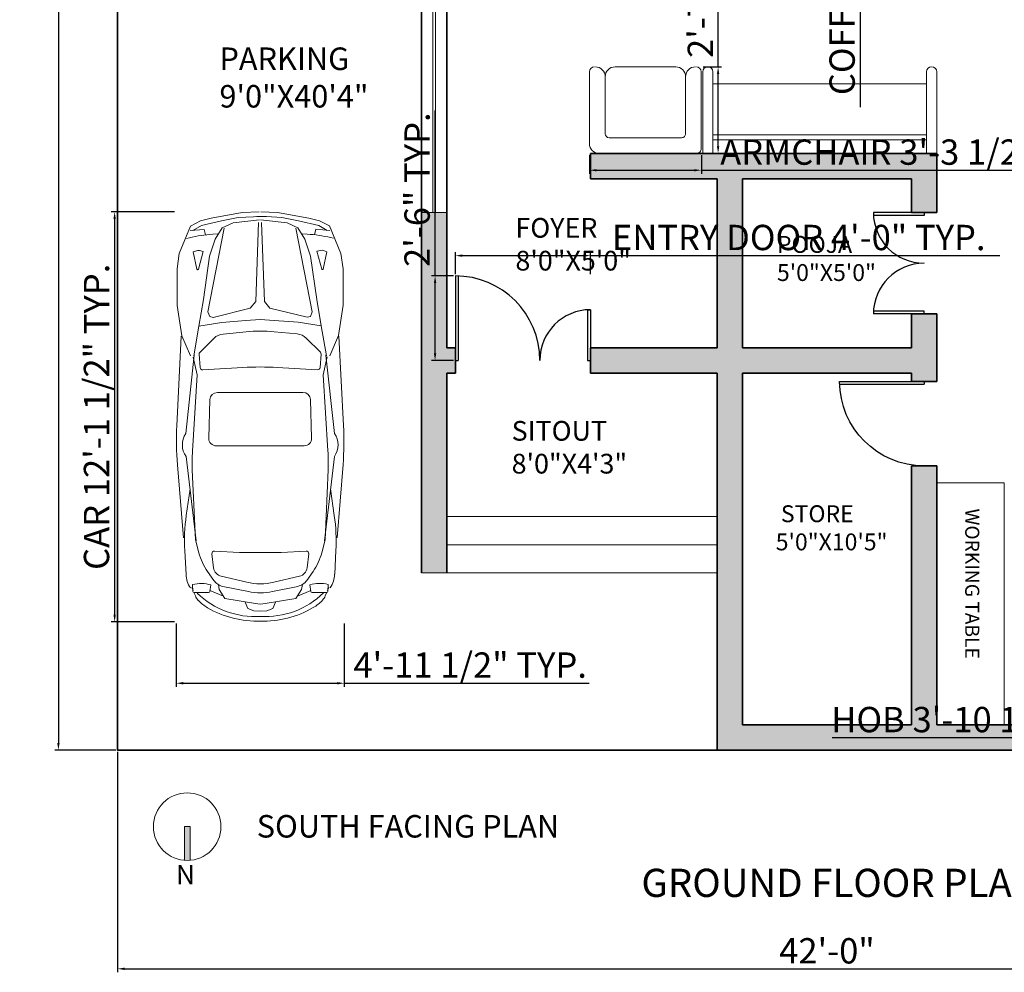
# Model space of a CAD drawing. Units: inches. Extents: x 4606 to 5879, y 1332 to 2209.
# Tile 1 of 7: x 4624 to 4974, y 1332 to 1671. Entities that reach past the tile are written whole.
import ezdxf

# ---------------------------------------------------------------- set-up
doc = ezdxf.new("R2010")
doc.units = ezdxf.units.IN
for name, color, linetype, lineweight in [('A-ANNO-DIMS', 2, 'Continuous', 18), ('A-ANNO-SYMB', 7, 'Continuous', 18), ('A-ANNO-TEXT', 7, 'Continuous', 18), ('A-ANNO-TITL', 7, 'Continuous', 25), ('A-AREA-IDEN', 7, 'Continuous', 18), ('A-DOOR', 4, 'Continuous', 25), ('A-FLOR-CASE', 32, 'Continuous', 18), ('A-FLOR-STRS', 7, 'Continuous', 20), ('A-FURN', 8, 'Continuous', 18), ('A-SITE-PARK', 8, 'Continuous', 13), ('A-WALL', 7, 'Continuous', 35), ('A-WALL-PATT', 252, 'Continuous', 13), ('window', 130, 'Continuous', 18)]:
    doc.layers.add(name, color=color, linetype=linetype, lineweight=lineweight)
doc.styles.get("Standard").update_dxf_attribs({"font": 'arial.ttf'})
doc.dimstyles.new('ISO-25', dxfattribs={"dimtxt": 9, "dimasz": 2.5, "dimexe": 1.25, "dimexo": 0.625, "dimtad": 1, "dimlunit": 3, "dimtxsty": 'Standard', "dimcen": 2.5, "dimadec": 0, "dimazin": 0, "dimtfac": 1, "dimtmove": 0, "dimatfit": 3, "dimfxl": 1, "dimarcsym": 0})

# ---------------------------------------------------------------- blocks, each defined once
blk = doc.blocks.new('D')
for p, q in [((0, 30), (0, 0)), ((1, 29.93), (1, 0)), ((47, 18), (47, 0)), ((47, 18), (48, 18)), ((48, 18), (48, 0)), ((0, 0), (1, 0)), ((47, 0), (48, 0))]:
    blk.add_line(p, q)
for centre, radius, start, end in [((0, 0), 30, 0, 90), ((48, 0), 18, 90, 180)]:
    blk.add_arc(centre, radius, start, end)
blk = doc.blocks.new('D3')
for p, q in [((0, 0), (0, 18)), ((1, 0), (1, 18)), ((35, 0), (35, 18)), ((36, 0), (36, 18)), ((0, 0), (1, 0)), ((36, 0), (35, 0))]:
    blk.add_line(p, q)
for centre, start, end in [((0, 0), 0, 90), ((36, 0), 90, 180)]:
    blk.add_arc(centre, 18, start, end)
blk = doc.blocks.new('sofa-27')
at = {"color": 0, "linetype": 'ByBlock'}
for p, q in [((-0.0591, 0.0591), (-0.0591, 0.4902)), ((0.0945, 0.5198), (0.459, 0.5198)), ((0.6125, 0.0295), (0.6125, 0.4902)), ((0.0354, 0.1181), (0.0354, 0.4607)), ((0.518, 0.1181), (0.518, 0.4607)), ((0.4944, 0.0945), (0.0591, 0.0945)), ((0.583, 0), (0, 0))]:
    blk.add_line(p, q, dxfattribs=at)
for centre, radius, start, end in [((-0.0295, 0.4902), 0.0295, 90, 180), ((-0.0236, 0.4607), 0.0591, 360, 90), ((0.0945, 0.4607), 0.0591, 90, 180), ((0.459, 0.4607), 0.0591, 0, 90), ((0.5771, 0.4607), 0.0591, 90, 180), ((0.583, 0.4902), 0.0295, 0, 90), ((0.0591, 0.1181), 0.0236, 180, 270), ((0.4944, 0.1181), 0.0236, 270, 0), ((0, 0.0591), 0.0591, 180, 270), ((0.583, 0.0295), 0.0295, 270, 0)]:
    blk.add_arc(centre, radius, start, end, dxfattribs=at)
blk = doc.blocks.new('A$C4A3239E3')
for p, q in [((1.2507, 1.6335), (2.1522, 1.6799)), ((1.4425, 1.5023), (2.2313, 1.5881)), ((2.4629, 1.587), (3.3117, 1.4863)), ((2.5445, 1.6742), (3.2816, 1.6148)), ((3.4104, 1.6024), (3.6491, 1.5899)), ((0.1359, 1.4288), (0.1867, 1.515)), ((0.1752, 1.399), (0.1867, 1.5408)), ((0.2661, 1.5794), (0.2592, 1.5495)), ((0.3898, 1.477), (0.4021, 1.5106)), ((0.4021, 1.5106), (0.5754, 1.4741)), ((1.4497, 1.5063), (1.149, 1.4553)), ((1.4612, 1.5146), (1.6407, 1.4739)), ((1.6407, 1.4739), (2.4076, 1.5225)), ((2.597, 1.5244), (3.3012, 1.4943)), ((2.7875, 1.5463), (3.0567, 1.5859)), ((3.3012, 1.4943), (3.4322, 1.4598)), ((3.8218, 1.5205), (3.7519, 1.525)), ((3.7813, 1.5317), (3.8128, 1.5185)), ((3.8334, 1.3629), (3.8334, 1.5081)), ((3.8376, 1.5081), (3.8668, 1.4958)), ((0.0905, 1.2265), (0.1359, 1.4288)), ((0.2308, 1.3867), (0.1752, 1.399)), ((0.3963, 1.4117), (0.388, 1.4492)), ((0.5758, 1.4596), (0.3963, 1.4117)), ((1.2717, 1.3033), (1.4134, 1.4465)), ((1.4329, 1.4538), (1.567, 1.4437)), ((1.59, 1.4175), (1.5668, 1.0125)), ((0.224, 1.314), (0.2207, 1.2655)), ((1.8899, 1.3452), (2.2788, 1.3576)), ((3.4158, 1.3024), (3.4294, 1.0516)), ((3.4434, 1.3284), (3.584, 1.3121)), ((3.6217, 1.372), (3.7108, 1.3099)), ((3.7558, 1.3393), (3.8231, 1.3506)), ((3.8137, 1.3503), (3.8686, 1.2144)), ((0.0565, 1.0588), (0.0905, 1.2265)), ((1.2074, 0.9801), (1.2293, 1.2125)), ((1.8186, 0.4085), (1.8178, 1.2708)), ((2.3557, 1.283), (2.3566, 0.3973)), ((3.6693, 1.236), (3.7299, 0.9762)), ((3.7535, 1.2644), (3.8014, 1.2553)), ((3.7713, 1.2181), (3.8245, 0.9626)), ((3.8014, 1.2553), (3.8941, 1.199)), ((3.8941, 1.199), (3.9452, 0.89)), ((0.0481, 0.9038), (0.0565, 1.0588)), ((3.4294, 1.0516), (3.4292, 0.8428)), ((3.9292, 0.9941), (3.9933, 0.9668)), ((3.9933, 0.9668), (4.0172, 0.906)), ((4.0172, 0.906), (4.0211, 0.842)), ((3.4299, 0.6309), (3.4292, 0.8396)), ((3.8948, 0.4844), (3.9453, 0.7934)), ((4.0174, 0.7775), (4.0211, 0.8416)), ((0.0482, 0.7723), (0.0569, 0.6172)), ((1.2077, 0.6979), (1.23, 0.4656)), ((3.6701, 0.4469), (3.7301, 0.7068)), ((3.772, 0.465), (3.8248, 0.7206)), ((3.9295, 0.6893), (3.9936, 0.7167)), ((3.9936, 0.7167), (4.0174, 0.7775)), ((0.0569, 0.6172), (0.0912, 0.4496)), ((1.5911, 0.2613), (1.5671, 0.6662)), ((3.4167, 0.38), (3.4299, 0.6309)), ((0.0912, 0.4496), (0.1371, 0.2474)), ((0.2249, 0.3624), (0.2215, 0.4109)), ((3.7543, 0.4187), (3.8022, 0.4279)), ((3.8022, 0.4279), (3.8948, 0.4844)), ((3.8147, 0.3328), (3.8693, 0.4688)), ((1.2726, 0.3749), (1.4146, 0.232)), ((1.8909, 0.3342), (2.2798, 0.3226)), ((3.4444, 0.354), (3.585, 0.3707)), ((3.6228, 0.3107), (3.7117, 0.3731)), ((3.7568, 0.3438), (3.8241, 0.3326)), ((3.8345, 0.3203), (3.8347, 0.1751)), ((0.1371, 0.2474), (0.188, 0.1613)), ((0.2318, 0.2897), (0.1763, 0.2773)), ((0.1763, 0.2773), (0.1881, 0.1355)), ((0.3975, 0.2651), (0.3892, 0.2275)), ((0.3911, 0.1998), (0.4034, 0.1661)), ((0.5771, 0.2174), (0.3975, 0.2651)), ((0.4034, 0.1661), (0.5767, 0.203)), ((1.451, 0.1722), (1.1502, 0.2226)), ((1.4341, 0.2247), (1.5682, 0.235)), ((1.4625, 0.1639), (1.6419, 0.205)), ((1.6419, 0.205), (2.4089, 0.1579)), ((3.3024, 0.1879), (3.4334, 0.2226)), ((0.2676, 0.0971), (0.2606, 0.127)), ((1.4438, 0.1762), (2.2328, 0.0919)), ((2.4644, 0.0936), (3.313, 0.1959)), ((2.5984, 0.1564), (3.3024, 0.1879)), ((2.7889, 0.1349), (3.0581, 0.0958)), ((3.8231, 0.1627), (3.7532, 0.1581)), ((3.7826, 0.1514), (3.8141, 0.1647)), ((3.8389, 0.1752), (3.8681, 0.1875)), ((1.2522, 0.0446), (2.1538, 0)), ((2.5461, 0.0065), (3.2831, 0.0673)), ((3.4119, 0.0799), (3.6506, 0.0929))]:
    blk.add_line(p, q)
for points in [[(0, 0.8478), (0.0053, 1.0159), (0.0622, 1.3298), (0.0905, 1.4375), (0.1412, 1.5365), (0.4188, 1.6529), (0.572, 1.6743), (0.9399, 1.6743), (1.2458, 1.627), (1.4497, 1.5408)], [(0.0815, 0.8439), (0.1088, 1.11), (0.1609, 1.2182), (0.2737, 1.2906), (0.4463, 1.3472), (0.8811, 1.4091), (1.149, 1.4553), (1.1121, 1.224), (1.0933, 0.9813), (1.085, 0.8389)], [(0.1644, 1.198), (1.0072, 1.3636), (1.0537, 1.3462), (1.0619, 1.3117), (0.9706, 0.937), (0.9035, 0.8818), (0.106, 0.853)], [(0, 0.8281), (0.0056, 0.6601), (0.0632, 0.3462), (0.0916, 0.2386), (0.1426, 0.1398), (0.4204, 0.0239), (0.5737, 0.0028), (0.9415, 0.0032), (1.2473, 0.0511), (1.4511, 0.1377)], [(0.0815, 0.8322), (0.1094, 0.5662), (0.1616, 0.4581), (0.2746, 0.3859), (0.4473, 0.3296), (0.8822, 0.2683), (1.1502, 0.2226), (1.1128, 0.4539), (1.0936, 0.6965), (1.085, 0.8389)], [(0.1651, 0.4782), (1.0082, 0.314), (1.0547, 0.3316), (1.0628, 0.366), (0.9708, 0.7406), (0.9036, 0.7957), (0.1061, 0.8232)]]:
    blk.add_lwpolyline(points)
for centre, radius, start, end in [((2.3053, -1.296), 2.9798, 85.39524, 92.94517), ((2.3463, 1.4226), 0.2016, 54.64918, 124.77695), ((3.3168, -0.183), 1.7879, 86.99981, 98.3676), ((3.6355, 1.3122), 0.278, 57.32995, 87.18237), ((1.7104, 1.2122), 1.4899, 166.91658, 176.08111), ((2.5206, -0.2618), 1.7879, 87.54913, 93.62371), ((4.0973, 1.4394), 0.3558, 166.09608, 196.35351), ((3.821, 1.5081), 0.0124, 0, 86.33043), ((3.8091, 1.3584), 0.149, 46.38363, 67.20138), ((0.4365, 1.46), 0.0497, 159.97873, 192.53841), ((0.5739, 1.4668), 0.00745, 284.96001, 78.11246), ((1.431, 1.429), 0.0248, 85.71507, 135.30465), ((1.5652, 1.4189), 0.0248, 356.72561, 85.71507), ((3.2805, 0.8834), 0.596, 55.07004, 75.25506), ((3.2466, 0.8963), 0.8285, 356.24509, 44.51945), ((3.6181, 1.158), 0.4258, 30.45768, 46.38363), ((1.3776, 1.1985), 0.149, 135.30465, 174.62136), ((1.8923, 1.2708), 0.0745, 91.82012, 179.9989), ((2.2812, 1.2831), 0.0745, 359.92446, 91.82012), ((3.4406, 1.3037), 0.0248, 83.37601, 183.11504), ((3.5726, 1.2134), 0.0993, 13.12265, 83.37601), ((3.6254, 1.1877), 0.149, 11.76937, 55.07004), ((3.821, 1.3629), 0.0124, 279.60772, 0), ((3.1325, 0.8724), 0.9892, 358.06945, 30.45768), ((4.5417, 0.8423), 2.9798, 176.72561, 183.38736), ((1.2382, 0.8392), 1.1919, 176.89416, 183.21881), ((2.6908, 0.8405), 1.4899, 174.62136, 185.49162), ((3.1495, 0.8409), 0.596, 346.99033, 13.12265), ((3.2411, 0.841), 0.596, 348.3436, 11.76937), ((3.2467, 0.7858), 0.8285, 315.59352, 3.86789), ((3.6512, 0.8414), 0.298, 350.72464, 9.38834), ((3.1326, 0.8094), 0.9892, 329.65529, 2.04353), ((1.3783, 0.4799), 0.149, 185.49162, 224.80833), ((1.8931, 0.4086), 0.0745, 180.11408, 268.29286), ((2.2821, 0.397), 0.0745, 268.29286, 0.18852), ((3.5733, 0.4693), 0.0993, 276.73697, 346.99033), ((3.6261, 0.4951), 0.149, 305.04293, 348.3436), ((1.7111, 0.4671), 1.4899, 184.03187, 193.1964), ((3.4415, 0.3787), 0.0248, 176.99794, 276.73697), ((3.2806, 0.7987), 0.596, 284.85791, 305.04293), ((4.0985, 0.2443), 0.3558, 163.75946, 194.01689), ((3.822, 0.3203), 0.0124, 0.11298, 80.50526), ((3.6188, 0.5248), 0.4258, 313.72935, 329.65529), ((0.4377, 0.2169), 0.0497, 167.57457, 200.13424), ((0.5752, 0.2102), 0.00745, 282.00051, 75.15297), ((1.4322, 0.2495), 0.0248, 224.80833, 274.3979), ((1.5663, 0.2598), 0.0248, 274.3979, 3.38736), ((3.8101, 0.3247), 0.149, 292.9116, 313.72935), ((2.5184, 1.9425), 1.7879, 266.48926, 272.56385), ((3.6364, 0.3706), 0.278, 272.9306, 302.78303), ((3.8223, 0.1751), 0.0124, 273.78255, 0.11298), ((2.3011, 2.9762), 2.9798, 267.1678, 274.71773), ((2.3474, 0.2577), 0.2016, 235.33603, 305.46379), ((3.3148, 1.8652), 1.7879, 261.74537, 273.11317)]:
    blk.add_arc(centre, radius, start, end)
blk = doc.blocks.new('D2')
for p, q in [((0, 30), (0, 0)), ((1, 30), (1, 0)), ((0, 0), (1, 0))]:
    blk.add_line(p, q)
blk.add_arc((0, 0), 30, 0, 90)
blk = doc.blocks.new('*D24')
at = {"layer": 'A-ANNO-DIMS', "color": 0, "lineweight": -2, "transparency": 16777216}
for p, q in [((4658.23, 2081.24), (4636.6, 2081.24)), ((4637.85, 2078.74), (4637.85, 1413.74)), ((4658.23, 1411.24), (4636.6, 1411.24))]:
    blk.add_line(p, q, dxfattribs=at)
at = {"layer": 'A-ANNO-DIMS', "color": 0, "transparency": 16777216}
for points in [[(4637.43, 2078.74), (4638.26, 2078.74), (4637.85, 2081.24)], [(4637.43, 1413.74), (4638.26, 1413.74), (4637.85, 1411.24)]]:
    blk.add_solid(points, dxfattribs=at)
at = {"layer": 'Defpoints', "color": 0, "transparency": 16777216}
for p in [(4658.85, 2081.24), (4637.85, 1411.24), (4658.85, 1411.24)]:
    blk.add_point(p, dxfattribs=at)
at = {"layer": 'A-ANNO-DIMS', "color": 0, "transparency": 16777216, "insert": (4632.62, 1746.24), "char_height": 9, "attachment_point": 5, "rotation": 90}
blk.add_mtext('55\'-10"', dxfattribs=at)
blk = doc.blocks.new('GLAZING-72IN')
for p, q in [((0, 0), (0, 72)), ((1, 0), (1, 72))]:
    blk.add_line(p, q)
blk = doc.blocks.new('NORTH-ARROW')
at = {"transparency": 33554687}
h = blk.add_hatch(color=256, dxfattribs=at)
h.dxf.hatch_style = 1
h.paths.add_polyline_path([(13, 20.5), (11, 20.5), (11, 8.55, 0.020861), (12, 8.5, 0.020861), (13, 8.55)])
for p, q in [((11, 8.5), (11, 20.5)), ((11, 20.5), (13, 20.5)), ((13, 20.5), (13, 8.55))]:
    blk.add_line(p, q)
blk.add_circle((12, 20.5), 12)
blk.add_text('N', height=6.9).set_placement((7.98, 0))
blk = doc.blocks.new('*D77')
at = {"layer": 'A-ANNO-DIMS', "color": 0, "lineweight": -2, "transparency": 16777216}
for p, q in [((4778.85, 1580.36), (4778.85, 1588.19)), ((4826.85, 1580.36), (4826.85, 1588.19)), ((4781.35, 1586.94), (4824.35, 1586.94)), ((4826.85, 1586.94), (4972.3, 1586.94))]:
    blk.add_line(p, q, dxfattribs=at)
at = {"layer": 'A-ANNO-DIMS', "color": 0, "transparency": 16777216}
for points in [[(4781.35, 1587.36), (4781.35, 1586.52), (4778.85, 1586.94)], [(4824.35, 1587.36), (4824.35, 1586.52), (4826.85, 1586.94)]]:
    blk.add_solid(points, dxfattribs=at)
at = {"layer": 'Defpoints', "color": 0, "transparency": 16777216}
for p in [(4826.85, 1586.94), (4778.85, 1579.74), (4826.85, 1579.74)]:
    blk.add_point(p, dxfattribs=at)
at = {"layer": 'A-ANNO-DIMS', "color": 0, "transparency": 16777216, "insert": (4900.83, 1592.22), "char_height": 9, "attachment_point": 5}
blk.add_mtext('ENTRY DOOR 4\'-0" TYP.', dxfattribs=at)
blk = doc.blocks.new('*D78')
at = {"layer": 'A-ANNO-DIMS', "color": 0, "lineweight": -2, "transparency": 16777216}
for p, q in [((4771.65, 1579.74), (4771.65, 1638.5)), ((4778.23, 1579.74), (4770.4, 1579.74)), ((4771.65, 1552.24), (4771.65, 1577.24)), ((4778.23, 1549.74), (4770.4, 1549.74))]:
    blk.add_line(p, q, dxfattribs=at)
at = {"layer": 'A-ANNO-DIMS', "color": 0, "transparency": 16777216}
for points in [[(4771.23, 1577.24), (4772.07, 1577.24), (4771.65, 1579.74)], [(4771.23, 1552.24), (4772.07, 1552.24), (4771.65, 1549.74)]]:
    blk.add_solid(points, dxfattribs=at)
at = {"layer": 'Defpoints', "color": 0, "transparency": 16777216}
for p in [(4771.65, 1579.74), (4778.85, 1579.74), (4778.85, 1549.74)]:
    blk.add_point(p, dxfattribs=at)
at = {"layer": 'A-ANNO-DIMS', "color": 0, "transparency": 16777216, "insert": (4766.43, 1610.37), "char_height": 9, "attachment_point": 5, "rotation": 90}
blk.add_mtext('2\'-6" TYP.', dxfattribs=at)
blk = doc.blocks.new('*D87')
at = {"layer": 'A-ANNO-DIMS', "color": 0, "lineweight": -2, "transparency": 16777216}
for p, q in [((4826.48, 1622.61), (4826.48, 1616.03)), ((4866.23, 1622.61), (4866.23, 1616.03)), ((4828.98, 1617.28), (4863.73, 1617.28)), ((4866.23, 1617.28), (5016.88, 1617.28))]:
    blk.add_line(p, q, dxfattribs=at)
at = {"layer": 'A-ANNO-DIMS', "color": 0, "transparency": 16777216}
for points in [[(4828.98, 1617.69), (4828.98, 1616.86), (4826.48, 1617.28)], [(4863.73, 1617.69), (4863.73, 1616.86), (4866.23, 1617.28)]]:
    blk.add_solid(points, dxfattribs=at)
at = {"layer": 'Defpoints', "color": 0, "transparency": 16777216}
for p in [(4826.48, 1623.24), (4866.23, 1623.24), (4866.23, 1617.28)]:
    blk.add_point(p, dxfattribs=at)
at = {"layer": 'A-ANNO-DIMS', "color": 0, "transparency": 16777216, "insert": (4942.8, 1622.56), "char_height": 9, "attachment_point": 5}
blk.add_mtext('ARMCHAIR 3\'-3 1/2" TYP.', dxfattribs=at)
blk = doc.blocks.new('*D88')
at = {"layer": 'A-ANNO-DIMS', "color": 0, "lineweight": -2, "transparency": 16777216}
for p, q in [((4872.19, 1654), (4872.19, 1712.76)), ((4866.85, 1654), (4873.44, 1654)), ((4872.19, 1625.74), (4872.19, 1651.5)), ((4866.85, 1623.24), (4873.44, 1623.24))]:
    blk.add_line(p, q, dxfattribs=at)
at = {"layer": 'A-ANNO-DIMS', "color": 0, "transparency": 16777216}
for points in [[(4871.77, 1651.5), (4872.6, 1651.5), (4872.19, 1654)], [(4871.77, 1625.74), (4872.6, 1625.74), (4872.19, 1623.24)]]:
    blk.add_solid(points, dxfattribs=at)
at = {"layer": 'Defpoints', "color": 0, "transparency": 16777216}
for p in [(4866.23, 1654), (4872.19, 1654), (4866.23, 1623.24)]:
    blk.add_point(p, dxfattribs=at)
at = {"layer": 'A-ANNO-DIMS', "color": 0, "transparency": 16777216, "insert": (4867.04, 1684.63), "char_height": 9, "attachment_point": 5, "rotation": 90}
blk.add_mtext('2\'-7" TYP.', dxfattribs=at)
blk = doc.blocks.new('*D103')
at = {"layer": 'A-ANNO-DIMS', "color": 0, "lineweight": -2, "transparency": 16777216}
for p, q in [((4679.05, 1602.48), (4656.58, 1602.48)), ((4657.83, 1599.98), (4657.83, 1459.37)), ((4679.05, 1456.87), (4656.58, 1456.87))]:
    blk.add_line(p, q, dxfattribs=at)
at = {"layer": 'A-ANNO-DIMS', "color": 0, "transparency": 16777216}
for points in [[(4657.41, 1599.98), (4658.25, 1599.98), (4657.83, 1602.48)], [(4657.41, 1459.37), (4658.25, 1459.37), (4657.83, 1456.87)]]:
    blk.add_solid(points, dxfattribs=at)
at = {"layer": 'Defpoints', "color": 0, "transparency": 16777216}
for p in [(4679.67, 1602.48), (4657.83, 1456.87), (4679.67, 1456.87)]:
    blk.add_point(p, dxfattribs=at)
at = {"layer": 'A-ANNO-DIMS', "color": 0, "transparency": 16777216, "insert": (4652.55, 1529.68), "char_height": 9, "attachment_point": 5, "rotation": 90}
blk.add_mtext('CAR 12\'-1 1/2" TYP.', dxfattribs=at)
blk = doc.blocks.new('*D104')
at = {"layer": 'A-ANNO-DIMS', "color": 0, "lineweight": -2, "transparency": 16777216}
for p, q in [((4679.67, 1456.25), (4679.67, 1433.78)), ((4739.4, 1456.25), (4739.4, 1433.78)), ((4682.17, 1435.03), (4736.9, 1435.03)), ((4739.4, 1435.03), (4826.33, 1435.03))]:
    blk.add_line(p, q, dxfattribs=at)
at = {"layer": 'A-ANNO-DIMS', "color": 0, "transparency": 16777216}
for points in [[(4682.17, 1435.45), (4682.17, 1434.61), (4679.67, 1435.03)], [(4736.9, 1435.45), (4736.9, 1434.61), (4739.4, 1435.03)]]:
    blk.add_solid(points, dxfattribs=at)
at = {"layer": 'Defpoints', "color": 0, "transparency": 16777216}
for p in [(4679.67, 1456.87), (4739.4, 1456.87), (4739.4, 1435.03)]:
    blk.add_point(p, dxfattribs=at)
at = {"layer": 'A-ANNO-DIMS', "color": 0, "transparency": 16777216, "insert": (4784.11, 1440.31), "char_height": 9, "attachment_point": 5}
blk.add_mtext('4\'-11 1/2" TYP.', dxfattribs=at)
blk = doc.blocks.new('*D105')
at = {"layer": 'A-ANNO-DIMS', "color": 0, "lineweight": -2, "transparency": 16777216}
for p, q in [((4927.48, 1801.23), (4921.43, 1801.23)), ((4922.68, 1798.73), (4922.68, 1767.59)), ((4927.48, 1765.09), (4921.43, 1765.09)), ((4922.68, 1765.09), (4922.68, 1639.71))]:
    blk.add_line(p, q, dxfattribs=at)
at = {"layer": 'A-ANNO-DIMS', "color": 0, "transparency": 16777216}
for points in [[(4922.27, 1798.73), (4923.1, 1798.73), (4922.68, 1801.23)], [(4922.27, 1767.59), (4923.1, 1767.59), (4922.68, 1765.09)]]:
    blk.add_solid(points, dxfattribs=at)
at = {"layer": 'Defpoints', "color": 0, "transparency": 16777216}
for p in [(4928.1, 1801.23), (4922.68, 1765.09), (4928.1, 1765.09)]:
    blk.add_point(p, dxfattribs=at)
at = {"layer": 'A-ANNO-DIMS', "color": 0, "transparency": 16777216, "insert": (4917.4, 1701.15), "char_height": 9, "attachment_point": 5, "rotation": 90}
blk.add_mtext('COFFEE TABLE 3\'-0"', dxfattribs=at)
blk = doc.blocks.new('*D109')
at = {"layer": 'A-ANNO-DIMS', "color": 0, "lineweight": -2, "transparency": 16777216}
for p, q in [((4998.57, 1422), (4998.57, 1414.41)), ((5045.02, 1422), (5045.02, 1414.41)), ((4998.57, 1415.66), (4912.68, 1415.66)), ((5042.52, 1415.66), (5001.07, 1415.66))]:
    blk.add_line(p, q, dxfattribs=at)
at = {"layer": 'A-ANNO-DIMS', "color": 0, "transparency": 16777216}
for points in [[(5001.07, 1416.08), (5001.07, 1415.25), (4998.57, 1415.66)], [(5042.52, 1416.08), (5042.52, 1415.25), (5045.02, 1415.66)]]:
    blk.add_solid(points, dxfattribs=at)
at = {"layer": 'Defpoints', "color": 0, "transparency": 16777216}
for p in [(4998.57, 1422.63), (5045.02, 1422.63), (4998.57, 1415.66)]:
    blk.add_point(p, dxfattribs=at)
at = {"layer": 'A-ANNO-DIMS', "color": 0, "transparency": 16777216, "insert": (4954.38, 1420.95), "char_height": 9, "attachment_point": 5}
blk.add_mtext('HOB 3\'-10 1/2"', dxfattribs=at)
blk = doc.blocks.new('*D113')
at = {"layer": 'A-ANNO-DIMS', "color": 0, "lineweight": -2, "transparency": 16777216}
for p, q in [((4658.85, 1410.61), (4658.85, 1332.33)), ((5162.85, 1410.61), (5162.85, 1332.33)), ((4661.35, 1333.58), (5160.35, 1333.58))]:
    blk.add_line(p, q, dxfattribs=at)
at = {"layer": 'A-ANNO-DIMS', "color": 0, "transparency": 16777216}
for points in [[(4661.35, 1334), (4661.35, 1333.16), (4658.85, 1333.58)], [(5160.35, 1334), (5160.35, 1333.16), (5162.85, 1333.58)]]:
    blk.add_solid(points, dxfattribs=at)
at = {"layer": 'Defpoints', "color": 0, "transparency": 16777216}
for p in [(4658.85, 1411.24), (5162.85, 1411.24), (5162.85, 1333.58)]:
    blk.add_point(p, dxfattribs=at)
at = {"layer": 'A-ANNO-DIMS', "color": 0, "transparency": 16777216, "insert": (4910.85, 1338.8), "char_height": 9, "attachment_point": 5}
blk.add_mtext('42\'-0"', dxfattribs=at)

msp = doc.modelspace()

# ---------------------------------------------------------------- hatches: boundary and pattern name
at = {"layer": 'A-WALL-PATT', "transparency": 33554687}
h = msp.add_hatch(color=256, dxfattribs=at)
h.dxf.hatch_style = 1
h.paths.add_polyline_path([(4715.85, 2081.239), (4658.85, 2081.239), (4658.85, 2054.239), (4667.85, 2054.239), (4667.85, 2072.239), (4715.85, 2072.239)])
h.paths.add_polyline_path([(4868.85, 2081.239), (4787.85, 2081.239), (4787.85, 2072.239), (4835.85, 2072.239), (4835.85, 1955.239), (4844.85, 1955.239), (4844.85, 1970.239), (4850.85, 1970.239), (4850.85, 1976.239), (4844.85, 1976.239), (4844.85, 2072.239), (4868.85, 2072.239)])
h.paths.add_polyline_path([(4940.85, 2081.239), (4892.85, 2081.239), (4892.85, 2072.239), (4916.85, 2072.239), (4916.85, 1976.239), (4880.85, 1976.239), (4880.85, 1970.239), (4916.85, 1970.239), (4916.85, 1904.239), (4844.85, 1904.239), (4844.85, 1925.239), (4835.85, 1925.239), (4835.85, 1904.239), (4832.85, 1904.239), (4832.85, 1895.239), (4919.85, 1895.239), (4991.85, 1895.239), (4991.85, 1904.239), (4988.85, 1904.239), (4988.85, 1925.239), (4982.85, 1925.239), (4982.85, 1904.239), (4922.85, 1904.239), (4922.85, 1970.239), (4946.85, 1970.239), (4946.85, 1976.239), (4922.85, 1976.239), (4922.85, 2072.239), (4940.85, 2072.239)])
h.paths.add_polyline_path([(5021.85, 2081.239), (4964.85, 2081.239), (4964.85, 2072.239), (4982.85, 2072.239), (4982.85, 1976.239), (4976.85, 1976.239), (4976.85, 1970.239), (4982.85, 1970.239), (4982.85, 1955.239), (4988.85, 1955.239), (4988.85, 2072.239), (5021.85, 2072.239)])
h.paths.add_polyline_path([(5135.85, 2081.239), (5093.85, 2081.239), (5093.85, 2072.239), (5126.85, 2072.239), (5126.85, 2054.239), (5135.85, 2054.239)])
h.paths.add_polyline_path([(5135.85, 2006.239), (5126.85, 2006.239), (5126.85, 1976.239), (5135.85, 1976.239)])
h.paths.add_polyline_path([(5135.85, 1928.239), (5126.85, 1928.239), (5126.85, 1904.239), (5027.85, 1904.239), (5027.85, 1895.239), (5126.85, 1895.239), (5126.85, 1871.239), (5135.85, 1871.239)])
h.paths.add_polyline_path([(4796.85, 1904.239), (4667.85, 1904.239), (4667.85, 1922.239), (4658.85, 1922.239), (4658.85, 1895.239), (4766.85, 1895.239), (4766.85, 1674.239), (4775.85, 1674.239), (4775.85, 1895.239), (4796.85, 1895.239)])
h.paths.add_polyline_path([(4667.85, 2006.239), (4658.85, 2006.239), (4658.85, 1970.239), (4667.85, 1970.239)])
h.paths.add_polyline_path([(4880.85, 1545.239), (4940.85, 1545.239), (4940.85, 1542.239), (4949.85, 1542.239), (4949.85, 1566.239), (4940.85, 1566.239), (4940.85, 1554.239), (4880.85, 1554.239), (4880.85, 1614.239), (4940.85, 1614.239), (4940.85, 1602.239), (4949.85, 1602.239), (4949.85, 1623.239), (4866.739, 1623.239), (4826.85, 1623.239), (4826.85, 1614.239), (4871.85, 1614.239), (4871.85, 1554.239), (4826.85, 1554.239), (4826.85, 1545.239), (4871.85, 1545.239), (4871.85, 1411.239), (4997.85, 1411.239), (4997.85, 1420.239), (4949.85, 1420.239), (4949.85, 1512.239), (4940.85, 1512.239), (4940.85, 1420.239), (4880.85, 1420.239)])
h.paths.add_polyline_path([(5102.85, 1446.239), (5093.85, 1446.239), (5093.85, 1420.239), (5045.85, 1420.239), (5045.85, 1411.239), (5102.85, 1411.239)])
h.paths.add_polyline_path([(5102.85, 1591.739), (5093.85, 1591.739), (5093.85, 1542.239), (5102.85, 1542.239)])
h.paths.add_polyline_path([(5135.85, 1691.239), (5126.85, 1691.239), (5126.85, 1673.239), (5030.85, 1673.239), (5030.85, 1676.239), (5021.85, 1676.239), (5021.85, 1673.239), (5003.85, 1673.239), (5003.85, 1664.239), (5093.85, 1664.239), (5093.85, 1639.739), (5102.85, 1639.739), (5102.85, 1664.239), (5135.85, 1664.239)])
h.paths.add_polyline_path([(5135.85, 1823.239), (5126.85, 1823.239), (5126.85, 1799.239), (5028.85, 1799.239), (5028.85, 1790.239), (5057.85, 1790.239), (5057.85, 1784.239), (5066.85, 1784.239), (5066.85, 1790.239), (5126.85, 1790.239), (5126.85, 1742.239), (5066.85, 1742.239), (5066.85, 1748.239), (5057.85, 1748.239), (5057.85, 1742.239), (5021.85, 1742.239), (5021.85, 1706.239), (5030.85, 1706.239), (5030.85, 1733.239), (5126.85, 1733.239), (5126.85, 1715.239), (5135.85, 1715.239)])
h.paths.add_polyline_path([(4775.85, 1602.239), (4766.85, 1602.239), (4766.85, 1474.239), (4775.85, 1474.239), (4775.85, 1545.239), (4778.85, 1545.239), (4778.85, 1554.239), (4775.85, 1554.239)])
h.paths.add_polyline_path([(4692.58, 1635.003), (4749.356, 1635.003), (4749.356, 1665.418), (4692.58, 1665.418)], flags=9)

# ---------------------------------------------------------------- linework, layer by layer
at = {"layer": 'A-FLOR-CASE'}
for q in [(4949.85, 1506.239), (4973.85, 1420.239)]:
    msp.add_line((4973.85, 1506.239), q, dxfattribs=at)
at = {"layer": 'A-FLOR-STRS'}
for p, q in [((4775.85, 1494.239), (4871.85, 1494.239)), ((4775.85, 1484.239), (4871.85, 1484.239)), ((4766.85, 1474.239), (4871.85, 1474.239))]:
    msp.add_line(p, q, dxfattribs=at)
at = {"layer": 'A-FURN'}
for p, q in [((4866.739, 1652.26), (4866.739, 1623.239)), ((4870.367, 1623.239), (4870.367, 1652.26)), ((4946.222, 1652.26), (4946.222, 1623.239)), ((4949.85, 1652.26), (4949.85, 1623.239)), ((4946.222, 1648.026), (4870.367, 1648.026)), ((4870.367, 1629.888), (4946.222, 1629.888)), ((4870.367, 1628.074), (4946.222, 1628.074)), ((4949.85, 1623.239), (4866.739, 1623.239))]:
    msp.add_line(p, q, dxfattribs=at)
for centre in [(4868.553, 1652.26), (4948.036, 1652.26)]:
    msp.add_arc(centre, 1.814, 0, 180, dxfattribs=at)
at = {"layer": 'A-WALL'}
for p, q in [((4766.85, 1895.239), (4766.85, 1474.239)), ((4775.85, 1895.239), (4775.85, 1554.239)), ((4826.85, 1623.239), (4949.85, 1623.239)), ((4826.85, 1623.239), (4826.85, 1614.239)), ((4949.85, 1623.239), (4949.85, 1602.239)), ((4826.85, 1614.239), (4871.85, 1614.239)), ((4871.85, 1614.239), (4871.85, 1554.239)), ((4880.85, 1614.239), (4880.85, 1554.239)), ((4880.85, 1614.239), (4940.85, 1614.239)), ((4940.85, 1614.239), (4940.85, 1602.239)), ((4940.85, 1602.239), (4949.85, 1602.239)), ((4940.85, 1566.239), (4949.85, 1566.239)), ((4940.85, 1566.239), (4940.85, 1554.239)), ((4949.85, 1566.239), (4949.85, 1542.239)), ((4775.85, 1554.239), (4778.85, 1554.239)), ((4778.85, 1554.239), (4778.85, 1545.239)), ((4826.85, 1554.239), (4871.85, 1554.239)), ((4826.85, 1554.239), (4826.85, 1545.239)), ((4880.85, 1554.239), (4940.85, 1554.239)), ((4775.85, 1545.239), (4778.85, 1545.239)), ((4775.85, 1545.239), (4775.85, 1474.239)), ((4826.85, 1545.239), (4871.85, 1545.239)), ((4871.85, 1545.239), (4871.85, 1411.239)), ((4880.85, 1545.239), (4940.85, 1545.239)), ((4880.85, 1545.239), (4880.85, 1420.239)), ((4940.85, 1545.239), (4940.85, 1542.239)), ((4940.85, 1542.239), (4949.85, 1542.239)), ((4940.85, 1512.239), (4949.85, 1512.239)), ((4940.85, 1512.239), (4940.85, 1420.239)), ((4949.85, 1512.239), (4949.85, 1420.239)), ((4880.85, 1420.239), (4940.85, 1420.239)), ((4949.85, 1420.239), (5093.85, 1420.239))]:
    msp.add_line(p, q, dxfattribs=at)
msp.add_lwpolyline([(5135.85, 1664.239), (5135.85, 2081.239), (4658.85, 2081.239), (4658.85, 1411.239), (5102.85, 1411.239)], dxfattribs=at)
at = {"layer": 'window'}
msp.add_line((4766.85, 1602.239), (4775.85, 1602.239), dxfattribs=at)

# ---------------------------------------------------------------- block references
at = {"layer": 'A-ANNO-SYMB'}
msp.add_blockref('NORTH-ARROW', (4671.599, 1363.576), dxfattribs=at)
at = {"layer": 'A-DOOR', "rotation": 90}
msp.add_blockref('D3', (4945.35, 1566.239), dxfattribs=at)
at = {"layer": 'A-DOOR'}
msp.add_blockref('D', (4778.85, 1549.739), dxfattribs=at)
at = {"layer": 'A-DOOR', "xscale": -1, "rotation": 90}
msp.add_blockref('D2', (4945.35, 1542.239), dxfattribs=at)
at = {"layer": 'A-FURN', "xscale": 59.17827105340016, "yscale": 59.17827105340016, "zscale": 59.17827105340016, "rotation": 359.9999999999668}
msp.add_blockref('sofa-27', (4829.977, 1623.239), dxfattribs=at)
at = {"layer": 'A-SITE-PARK', "xscale": 35.27598425228, "yscale": 35.27598425228, "zscale": 35.27598425228, "rotation": 270}
msp.add_blockref('A$C4A3239E3', (4679.899, 1602.485), dxfattribs=at)
at = {"layer": 'window'}
msp.add_blockref('GLAZING-72IN', (4770.85, 1602.239), dxfattribs=at)

# ---------------------------------------------------------------- texts
at = {"layer": 'A-ANNO-TEXT', "insert": (4964.957, 1497.095), "char_height": 5, "attachment_point": 1, "rotation": 270}
msp.add_mtext_dynamic_manual_height_columns('{\\fTimes New Roman|b0|i0|c0|p18;WORKING TABLE}', width=110.76054, gutter_width=12.5, heights=[0], dxfattribs=at)
at = {"layer": 'A-ANNO-TITL', "attachment_point": 1}
for s, insert, char_height in [('{\\fTimes New Roman|b0|i0|c0|p18;SOUTH FACING PLAN}', (4708.293, 1388.203), 8), ('{\\fTimes New Roman|b0|i0|c0|p18;GROUND FLOOR PLAN}', (4844.94, 1369.116), 10)]:
    msp.add_mtext_dynamic_manual_height_columns(s, width=196.26071, gutter_width=12.5, heights=[0], dxfattribs=dict(at, insert=insert, char_height=char_height))
at = {"layer": 'A-AREA-IDEN', "attachment_point": 1}
for s, width, insert, char_height in [('{\\fTimes New Roman|b0|i0|c0|p18;PARKING\\P9\'0"X40\'4"}', 110.76054, (4695.047, 1660.892), 8), ('{\\fTimes New Roman|b0|i0|c0|p18;FOYER\\P8\'0"X5\'0"}', 80.30411, (4800.195, 1600.32), 7), ('{\\fTimes New Roman|b0|i0|c0|p18;POOJA\\P5\'0"X5\'0"}', 80.30411, (4893.088, 1593.934), 6), ('{\\fTimes New Roman|b0|i0|c0|p18;SITOUT\\P8\'0"X4\'3"}', 80.30411, (4798.845, 1528.201), 7), ('{\\fTimes New Roman|b0|i0|c0|p18; STORE\\P5\'0"X10\'5"}', 80.30411, (4892.655, 1498.248), 6)]:
    msp.add_mtext_dynamic_manual_height_columns(s, width=width, gutter_width=12.5, heights=[0], dxfattribs=dict(at, insert=insert, char_height=char_height))

# ---------------------------------------------------------------- dimensions: what is measured, and where the dimension line sits
at = {"layer": 'A-ANNO-DIMS'}
dim = msp.add_linear_dim(base=(4637.845, 1411.239), p1=(4658.85, 2081.239), p2=(4658.85, 1411.239), angle=90, dimstyle='ISO-25', override={"dimclrd": 0, "dimclre": 0, "dimclrt": 0}, dxfattribs=at)
dim.commit()
dim.dimension.update_dxf_attribs({"geometry": '*D24', "text_midpoint": (4632.625, 1746.239)})
for base, p1, p2, angle, text, picture, middle in [((4922.684, 1765.092), (4928.104, 1801.225), (4928.104, 1765.092), 270, 'COFFEE TABLE <>', '*D105', (4917.399, 1701.153)), ((4872.186, 1653.997), (4866.225, 1623.239), (4866.225, 1653.997), 90, '<> TYP.', '*D88', (4867.04, 1684.628)), ((4771.65, 1579.739), (4778.85, 1549.739), (4778.85, 1579.739), 90, '<> TYP.', '*D78', (4766.43, 1610.37)), ((4657.829, 1456.873), (4679.671, 1602.485), (4679.671, 1456.873), 270, 'CAR <> TYP.', '*D103', (4652.551, 1529.679)), ((4998.571, 1415.662), (5045.017, 1422.629), (4998.571, 1422.629), 180, 'HOB <>', '*D109', (4954.375, 1420.947))]:
    dim = msp.add_linear_dim(base=base, p1=p1, p2=p2, angle=angle, text=text, dimstyle='ISO-25', override={"dimdec": 1, "dimlfac": 1, "dimrnd": 0, "dimzin": 1, "dimdsep": 46, "dimlunit": 4, "dimfrac": 2}, dxfattribs=at)
    dim.commit()
    dim.dimension.update_dxf_attribs({"geometry": picture, "text_midpoint": middle})
for base, p1, p2, text, picture, middle in [((4866.225, 1617.277), (4826.482, 1623.239), (4866.225, 1623.239), 'ARMCHAIR <> TYP.', '*D87', (4942.802, 1622.559)), ((4826.85, 1586.939), (4778.85, 1579.739), (4826.85, 1579.739), 'ENTRY DOOR <> TYP.', '*D77', (4900.827, 1592.22)), ((4739.396, 1435.031), (4679.671, 1456.873), (4739.396, 1456.873), '<> TYP.', '*D104', (4784.114, 1440.309))]:
    dim = msp.add_linear_dim(base=base, p1=p1, p2=p2, text=text, dimstyle='ISO-25', override={"dimdec": 1, "dimlfac": 1, "dimrnd": 0, "dimzin": 1, "dimdsep": 46, "dimlunit": 4, "dimfrac": 2}, dxfattribs=at)
    dim.commit()
    dim.dimension.update_dxf_attribs({"geometry": picture, "text_midpoint": middle})
dim = msp.add_linear_dim(base=(5162.85, 1333.58), p1=(4658.85, 1411.239), p2=(5162.85, 1411.239), dimstyle='ISO-25', override={"dimdec": 1, "dimlfac": 1, "dimrnd": 0, "dimzin": 1, "dimdsep": 46, "dimlunit": 4, "dimfrac": 2}, dxfattribs=at)
dim.commit()
dim.dimension.update_dxf_attribs({"geometry": '*D113', "text_midpoint": (4910.85, 1338.8)})

doc.saveas('drawing.dxf')
